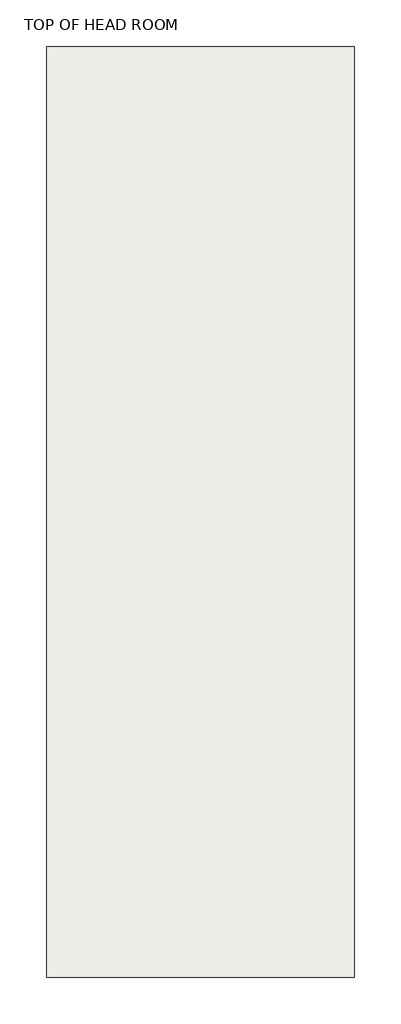
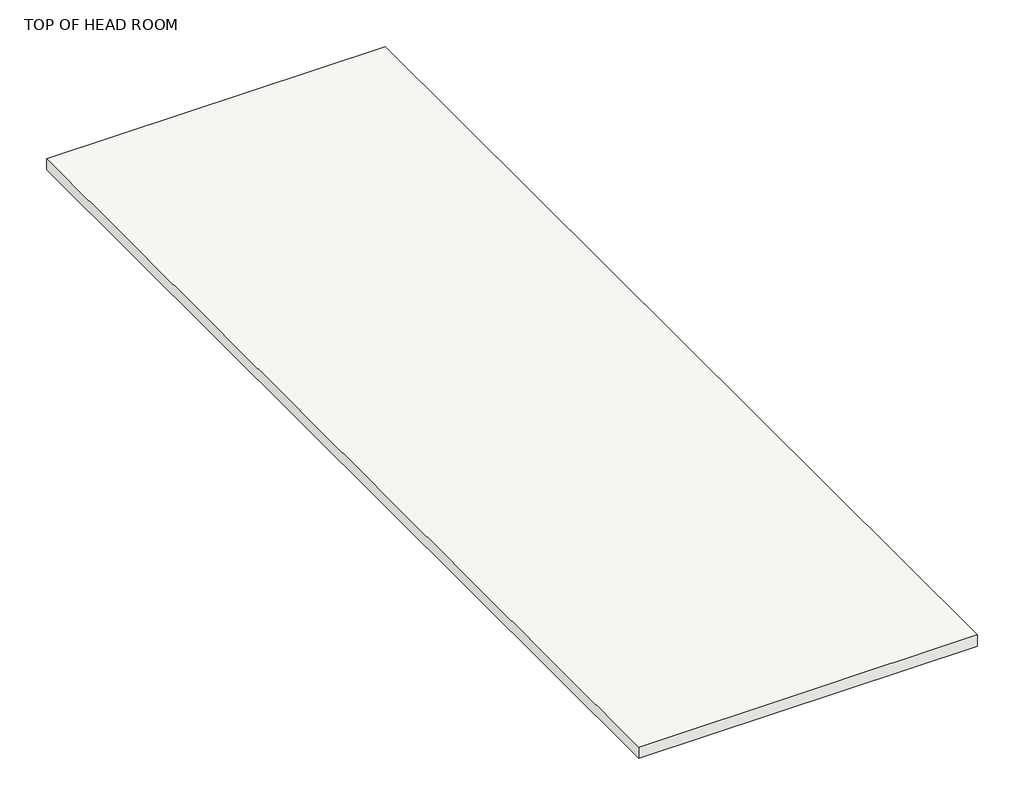
# One storey: 1 roof.
"""IFC4 building model written with IfcOpenShell, lengths in millimetres."""

from ifc_helpers import new_model, si_unit, frame, origin, place, context, project, spatial, polyline, outline, extrude, element, save

model = new_model("IFC4")

# Units and contexts
model_context = context("Model", 3, world=origin())
ifc_project = project(units=[si_unit("LENGTHUNIT", "METRE", prefix="MILLI")], contexts=[model_context])

# Site, building, storey
site = spatial("IfcSite", under=ifc_project)
building = spatial("IfcBuilding", under=site)
storey = spatial("IfcBuildingStorey", under=building, Name="TOP OF HEAD ROOM", Elevation=8534.4)

# Roof
placement = place(None, origin())
element("IfcRoof", 1, ObjectType="ROOFING 2", at=placement, inside=storey, context=model_context, shape_type="SweptSolid", body=[
    extrude(outline(polyline([(-12780.7206309, 4742.0155883), (-8443.9263881, 4742.0155883), (-8443.9263881, -8388.4150903), (-12780.7206309, -8388.4150903), (-12780.7206309, 4742.0155883)])), frame((0.0, 0.0, 8534.4), z_axis=(0.0, 0.0, 1.0), x_axis=(1.0, 0.0, 0.0)), (0.0, 0.0, 1.0), 152.4),
])

save(model, "model.ifc")

# Revit data of these elements
# Type "ROOFING 2"
#   Assembly Code = "B1020"
# Element 1 (IfcRoof, "ROOFING 2")
#   built-in parameter 1001705 = 28.5 (stored number, unit not read)
#   built-in parameter 1001710 = 33615
#   Phase Created = New Construction
